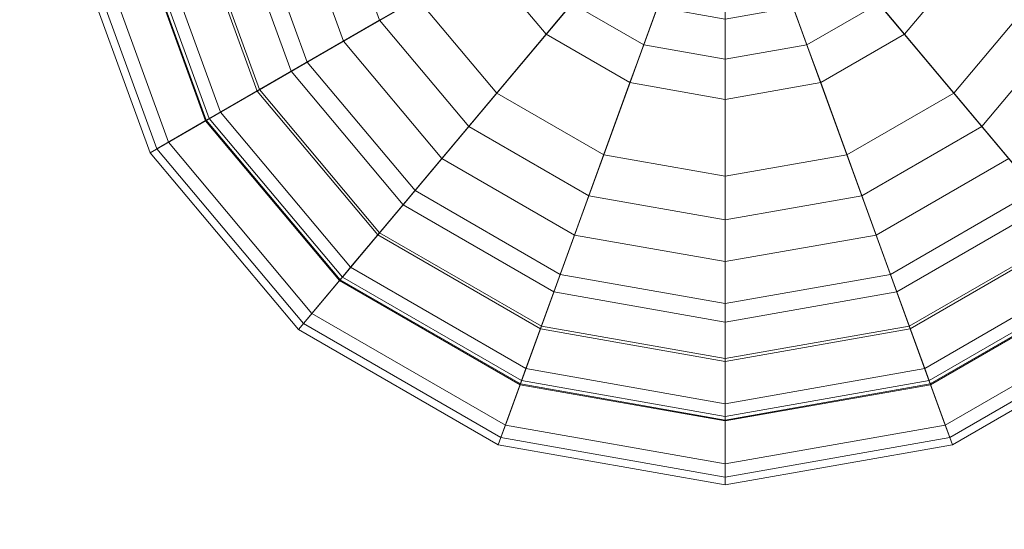
# Model space of a CAD drawing. Units: inches. Extents: x 375 to 1122, y 27 to 1069.
# Tile 90 of 155: x 728.243 to 730.25, y 859.033 to 860.072. Entities that reach past the tile are written whole.
import ezdxf

# ---------------------------------------------------------------- set-up
doc = ezdxf.new("R2010")
doc.units = ezdxf.units.IN
doc.layers.add('A-ANNO-DIMS', color=2, linetype='Continuous', lineweight=18)
doc.layers.add('Furniture', color=30, linetype='Continuous', lineweight=18)
doc.styles.get("Standard").update_dxf_attribs({"font": 'arial.ttf'})
doc.dimstyles.new('ISO-25', dxfattribs={"dimtxt": 12, "dimasz": 2.5, "dimexe": 1.5, "dimexo": 1.5, "dimtad": 1, "dimdec": 1, "dimlunit": 3, "dimtxsty": 'Standard', "dimblk": 'ARCHTICK', "dimcen": 2.5, "dimadec": 0, "dimazin": 0, "dimtfac": 1, "dimtdec": 1, "dimtmove": 0, "dimatfit": 3, "dimfxl": 1.5, "dimfxlon": 1, "dimarcsym": 0})

# ---------------------------------------------------------------- blocks, each defined once
blk = doc.blocks.new('A$C403C54AD')
for points in [[(1.963274, 1.147718, -0.060915), (1.946342, 1.118392, -0.057836), (1.946342, 1.118392, -0.057836), (1.952223, 1.15174, -0.060915)], [(1.95345, 1.130702, -0.054409), (1.961641, 1.144889, -0.057684), (1.951655, 1.148524, -0.057684), (1.948811, 1.13239, -0.054409)], [(1.972282, 1.140158, -0.060915), (1.946342, 1.118392, -0.057836), (1.946342, 1.118392, -0.057836), (1.963274, 1.147718, -0.060915)], [(1.957231, 1.127529, -0.054409), (1.969781, 1.138059, -0.057684), (1.961641, 1.144889, -0.057684), (1.95345, 1.130702, -0.054409)], [(1.96735, 1.13602, 0.042594), (1.961937, 1.131478, 0.032362), (1.956521, 1.136022, 0.032362), (1.960054, 1.142142, 0.042594)], [(1.978163, 1.129974, -0.060915), (1.946342, 1.118392, -0.057836), (1.946342, 1.118392, -0.057836), (1.972282, 1.140158, -0.060915)], [(1.975094, 1.128857, -0.057684), (1.978163, 1.129974, -0.060915), (1.972282, 1.140158, -0.060915), (1.969781, 1.138059, -0.057684)], [(1.960229, 1.130044, 0.03455), (1.965197, 1.134213, 0.043942), (1.958649, 1.139708, 0.043942), (1.955406, 1.134091, 0.03455)], [(1.975056, 1.128843, 0.102069), (1.977788, 1.129837, 0.088845), (1.971977, 1.139902, 0.088845), (1.96975, 1.138033, 0.102069)], [(1.977788, 1.129837, 0.088845), (1.977153, 1.129606, 0.060603), (1.97146, 1.139468, 0.060603), (1.971977, 1.139902, 0.088845)], [(1.977153, 1.129606, 0.060603), (1.972112, 1.127772, 0.042594), (1.96735, 1.13602, 0.042594), (1.97146, 1.139468, 0.060603)], [(1.956521, 1.136022, 0.032362), (1.951402, 1.127155, 0.024995), (1.9481, 1.128357, 0.024995), (1.949878, 1.13844, 0.032362)], [(1.9597, 1.123254, -0.054409), (1.975094, 1.128857, -0.057684), (1.969781, 1.138059, -0.057684), (1.957231, 1.127529, -0.054409)], [(1.970361, 1.127134, 0.111475), (1.975056, 1.128843, 0.102069), (1.96975, 1.138033, 0.102069), (1.965922, 1.134821, 0.111475)], [(1.974889, 1.128782, 0.088628), (1.972249, 1.127821, 0.101264), (1.967462, 1.136113, 0.101264), (1.969614, 1.137919, 0.088628)], [(1.974271, 1.128557, 0.061088), (1.974889, 1.128782, 0.088628), (1.969614, 1.137919, 0.088628), (1.96911, 1.137496, 0.061088)], [(1.969471, 1.12681, 0.043942), (1.974271, 1.128557, 0.061088), (1.96911, 1.137496, 0.061088), (1.965197, 1.134213, 0.043942)], [(1.972249, 1.127821, 0.101264), (1.967468, 1.126081, 0.111475), (1.963564, 1.132843, 0.111475), (1.967462, 1.136113, 0.101264)], [(1.961937, 1.131478, 0.032362), (1.954094, 1.124896, 0.024995), (1.951402, 1.127155, 0.024995), (1.956521, 1.136022, 0.032362)], [(1.972112, 1.127772, 0.042594), (1.965472, 1.125355, 0.032362), (1.961937, 1.131478, 0.032362), (1.96735, 1.13602, 0.042594)], [(1.967468, 1.126081, 0.111475), (1.970361, 1.127134, 0.111475), (1.965922, 1.134821, 0.111475), (1.963564, 1.132843, 0.111475)], [(1.953163, 1.124116, 0.027913), (1.960229, 1.130044, 0.03455), (1.955406, 1.134091, 0.03455), (1.950795, 1.126103, 0.027913)], [(1.963376, 1.124592, 0.03455), (1.969471, 1.12681, 0.043942), (1.965197, 1.134213, 0.043942), (1.960229, 1.130044, 0.03455)], [(1.965472, 1.125355, 0.032362), (1.955851, 1.121853, 0.024995), (1.954094, 1.124896, 0.024995), (1.961937, 1.131478, 0.032362)], [(1.955663, 1.126213, -0.051544), (1.957231, 1.127529, -0.054409), (1.95345, 1.130702, -0.054409), (1.952426, 1.128929, -0.051544)], [(1.980205, 1.118392, -0.060915), (1.946342, 1.118392, -0.057836), (1.946342, 1.118392, -0.057836), (1.978163, 1.129974, -0.060915)], [(1.95471, 1.121437, 0.027913), (1.963376, 1.124592, 0.03455), (1.960229, 1.130044, 0.03455), (1.953163, 1.124116, 0.027913)], [(1.979131, 1.118392, 0.060603), (1.973766, 1.118392, 0.042594), (1.972112, 1.127772, 0.042594), (1.977153, 1.129606, 0.060603)], [(1.976898, 1.118392, 0.102069), (1.979806, 1.118392, 0.088845), (1.977788, 1.129837, 0.088845), (1.975056, 1.128843, 0.102069)], [(1.976939, 1.118392, -0.057684), (1.980205, 1.118392, -0.060915), (1.978163, 1.129974, -0.060915), (1.975094, 1.128857, -0.057684)], [(1.979806, 1.118392, 0.088845), (1.979131, 1.118392, 0.060603), (1.977153, 1.129606, 0.060603), (1.977788, 1.129837, 0.088845)], [(1.960557, 1.118392, -0.054409), (1.976939, 1.118392, -0.057684), (1.975094, 1.128857, -0.057684), (1.9597, 1.123254, -0.054409)], [(1.971902, 1.118392, 0.111475), (1.976898, 1.118392, 0.102069), (1.975056, 1.128843, 0.102069), (1.970361, 1.127134, 0.111475)], [(1.976721, 1.118392, 0.088628), (1.973912, 1.118392, 0.101264), (1.972249, 1.127821, 0.101264), (1.974889, 1.128782, 0.088628)], [(1.976063, 1.118392, 0.061088), (1.976721, 1.118392, 0.088628), (1.974889, 1.128782, 0.088628), (1.974271, 1.128557, 0.061088)], [(1.970956, 1.118392, 0.043942), (1.976063, 1.118392, 0.061088), (1.974271, 1.128557, 0.061088), (1.969471, 1.12681, 0.043942)], [(1.973766, 1.118392, 0.042594), (1.9667, 1.118392, 0.032362), (1.965472, 1.125355, 0.032362), (1.972112, 1.127772, 0.042594)], [(1.973912, 1.118392, 0.101264), (1.968824, 1.118392, 0.111475), (1.967468, 1.126081, 0.111475), (1.972249, 1.127821, 0.101264)], [(1.957775, 1.122553, -0.051544), (1.9597, 1.123254, -0.054409), (1.957231, 1.127529, -0.054409), (1.955663, 1.126213, -0.051544)], [(1.968824, 1.118392, 0.111475), (1.971902, 1.118392, 0.111475), (1.970361, 1.127134, 0.111475), (1.967468, 1.126081, 0.111475)], [(1.96447, 1.118392, 0.03455), (1.970956, 1.118392, 0.043942), (1.969471, 1.12681, 0.043942), (1.963376, 1.124592, 0.03455)], [(1.953927, 1.121153, -0.049498), (1.957775, 1.122553, -0.051544), (1.955663, 1.126213, -0.051544), (1.952525, 1.12358, -0.049498)], [(1.9667, 1.118392, 0.032362), (1.956461, 1.118392, 0.024995), (1.955851, 1.121853, 0.024995), (1.965472, 1.125355, 0.032362)], [(1.955247, 1.118392, 0.027913), (1.96447, 1.118392, 0.03455), (1.963376, 1.124592, 0.03455), (1.95471, 1.121437, 0.027913)], [(1.958509, 1.118392, -0.051544), (1.960557, 1.118392, -0.054409), (1.9597, 1.123254, -0.054409), (1.957775, 1.122553, -0.051544)], [(1.954413, 1.118392, -0.049498), (1.958509, 1.118392, -0.051544), (1.957775, 1.122553, -0.051544), (1.953927, 1.121153, -0.049498)], [(1.972282, 1.096626, -0.060915), (1.946342, 1.118392, -0.057836), (1.946342, 1.118392, -0.057836), (1.978163, 1.106811, -0.060915)], [(1.963274, 1.089067, -0.060915), (1.946342, 1.118392, -0.057836), (1.946342, 1.118392, -0.057836), (1.972282, 1.096626, -0.060915)], [(1.952223, 1.085044, -0.060915), (1.946342, 1.118392, -0.057836), (1.946342, 1.118392, -0.057836), (1.963274, 1.089067, -0.060915)], [(1.978163, 1.106811, -0.060915), (1.946342, 1.118392, -0.057836), (1.946342, 1.118392, -0.057836), (1.980205, 1.118392, -0.060915)], [(1.953927, 1.115632, -0.049498), (1.957775, 1.114231, -0.051544), (1.958509, 1.118392, -0.051544), (1.954413, 1.118392, -0.049498)], [(1.95471, 1.115347, 0.027913), (1.963376, 1.112192, 0.03455), (1.96447, 1.118392, 0.03455), (1.955247, 1.118392, 0.027913)], [(1.965472, 1.111429, 0.032362), (1.955851, 1.114931, 0.024995), (1.956461, 1.118392, 0.024995), (1.9667, 1.118392, 0.032362)], [(1.957775, 1.114231, -0.051544), (1.9597, 1.113531, -0.054409), (1.960557, 1.118392, -0.054409), (1.958509, 1.118392, -0.051544)], [(1.9597, 1.113531, -0.054409), (1.975094, 1.107928, -0.057684), (1.976939, 1.118392, -0.057684), (1.960557, 1.118392, -0.054409)], [(1.963376, 1.112192, 0.03455), (1.969471, 1.109974, 0.043942), (1.970956, 1.118392, 0.043942), (1.96447, 1.118392, 0.03455)], [(1.972112, 1.109013, 0.042594), (1.965472, 1.111429, 0.032362), (1.9667, 1.118392, 0.032362), (1.973766, 1.118392, 0.042594)], [(1.967468, 1.110703, 0.111475), (1.970361, 1.10965, 0.111475), (1.971902, 1.118392, 0.111475), (1.968824, 1.118392, 0.111475)], [(1.972249, 1.108963, 0.101264), (1.967468, 1.110703, 0.111475), (1.968824, 1.118392, 0.111475), (1.973912, 1.118392, 0.101264)], [(1.969471, 1.109974, 0.043942), (1.974271, 1.108227, 0.061088), (1.976063, 1.118392, 0.061088), (1.970956, 1.118392, 0.043942)], [(1.970361, 1.10965, 0.111475), (1.975056, 1.107941, 0.102069), (1.976898, 1.118392, 0.102069), (1.971902, 1.118392, 0.111475)], [(1.977153, 1.107178, 0.060603), (1.972112, 1.109013, 0.042594), (1.973766, 1.118392, 0.042594), (1.979131, 1.118392, 0.060603)], [(1.974889, 1.108002, 0.088628), (1.972249, 1.108963, 0.101264), (1.973912, 1.118392, 0.101264), (1.976721, 1.118392, 0.088628)], [(1.974271, 1.108227, 0.061088), (1.974889, 1.108002, 0.088628), (1.976721, 1.118392, 0.088628), (1.976063, 1.118392, 0.061088)], [(1.975056, 1.107941, 0.102069), (1.977788, 1.106947, 0.088845), (1.979806, 1.118392, 0.088845), (1.976898, 1.118392, 0.102069)], [(1.975094, 1.107928, -0.057684), (1.978163, 1.106811, -0.060915), (1.980205, 1.118392, -0.060915), (1.976939, 1.118392, -0.057684)], [(1.977788, 1.106947, 0.088845), (1.977153, 1.107178, 0.060603), (1.979131, 1.118392, 0.060603), (1.979806, 1.118392, 0.088845)], [(1.952525, 1.113204, -0.049498), (1.955663, 1.110572, -0.051544), (1.957775, 1.114231, -0.051544), (1.953927, 1.115632, -0.049498)], [(1.953163, 1.112669, 0.027913), (1.960229, 1.10674, 0.03455), (1.963376, 1.112192, 0.03455), (1.95471, 1.115347, 0.027913)], [(1.961937, 1.105307, 0.032362), (1.954094, 1.111888, 0.024995), (1.955851, 1.114931, 0.024995), (1.965472, 1.111429, 0.032362)], [(1.955663, 1.110572, -0.051544), (1.957231, 1.109255, -0.054409), (1.9597, 1.113531, -0.054409), (1.957775, 1.114231, -0.051544)], [(1.957231, 1.109255, -0.054409), (1.969781, 1.098725, -0.057684), (1.975094, 1.107928, -0.057684), (1.9597, 1.113531, -0.054409)], [(1.950795, 1.110681, 0.027913), (1.955406, 1.102693, 0.03455), (1.960229, 1.10674, 0.03455), (1.953163, 1.112669, 0.027913)], [(1.960229, 1.10674, 0.03455), (1.965197, 1.102571, 0.043942), (1.969471, 1.109974, 0.043942), (1.963376, 1.112192, 0.03455)], [(1.956521, 1.100762, 0.032362), (1.951402, 1.109629, 0.024995), (1.954094, 1.111888, 0.024995), (1.961937, 1.105307, 0.032362)], [(1.96735, 1.100764, 0.042594), (1.961937, 1.105307, 0.032362), (1.965472, 1.111429, 0.032362), (1.972112, 1.109013, 0.042594)], [(1.952426, 1.107856, -0.051544), (1.95345, 1.106082, -0.054409), (1.957231, 1.109255, -0.054409), (1.955663, 1.110572, -0.051544)], [(1.963564, 1.103941, 0.111475), (1.965922, 1.101963, 0.111475), (1.970361, 1.10965, 0.111475), (1.967468, 1.110703, 0.111475)], [(1.967462, 1.100671, 0.101264), (1.963564, 1.103941, 0.111475), (1.967468, 1.110703, 0.111475), (1.972249, 1.108963, 0.101264)], [(1.949878, 1.098344, 0.032362), (1.9481, 1.108427, 0.024995), (1.951402, 1.109629, 0.024995), (1.956521, 1.100762, 0.032362)], [(1.965197, 1.102571, 0.043942), (1.96911, 1.099288, 0.061088), (1.974271, 1.108227, 0.061088), (1.969471, 1.109974, 0.043942)], [(1.965922, 1.101963, 0.111475), (1.96975, 1.098751, 0.102069), (1.975056, 1.107941, 0.102069), (1.970361, 1.10965, 0.111475)], [(1.95345, 1.106082, -0.054409), (1.961641, 1.091895, -0.057684), (1.969781, 1.098725, -0.057684), (1.957231, 1.109255, -0.054409)], [(1.97146, 1.097316, 0.060603), (1.96735, 1.100764, 0.042594), (1.972112, 1.109013, 0.042594), (1.977153, 1.107178, 0.060603)], [(1.969614, 1.098865, 0.088628), (1.967462, 1.100671, 0.101264), (1.972249, 1.108963, 0.101264), (1.974889, 1.108002, 0.088628)], [(1.96911, 1.099288, 0.061088), (1.969614, 1.098865, 0.088628), (1.974889, 1.108002, 0.088628), (1.974271, 1.108227, 0.061088)], [(1.96975, 1.098751, 0.102069), (1.971977, 1.096882, 0.088845), (1.977788, 1.106947, 0.088845), (1.975056, 1.107941, 0.102069)], [(1.969781, 1.098725, -0.057684), (1.972282, 1.096626, -0.060915), (1.978163, 1.106811, -0.060915), (1.975094, 1.107928, -0.057684)], [(1.971977, 1.096882, 0.088845), (1.97146, 1.097316, 0.060603), (1.977153, 1.107178, 0.060603), (1.977788, 1.106947, 0.088845)], [(1.955406, 1.102693, 0.03455), (1.958649, 1.097077, 0.043942), (1.965197, 1.102571, 0.043942), (1.960229, 1.10674, 0.03455)], [(1.948811, 1.104394, -0.054409), (1.951655, 1.088261, -0.057684), (1.961641, 1.091895, -0.057684), (1.95345, 1.106082, -0.054409)], [(1.960054, 1.094642, 0.042594), (1.956521, 1.100762, 0.032362), (1.961937, 1.105307, 0.032362), (1.96735, 1.100764, 0.042594)], [(1.957583, 1.098923, 0.111475), (1.959122, 1.096257, 0.111475), (1.965922, 1.101963, 0.111475), (1.963564, 1.103941, 0.111475)], [(1.960127, 1.094517, 0.101264), (1.957583, 1.098923, 0.111475), (1.963564, 1.103941, 0.111475), (1.967462, 1.100671, 0.101264)], [(1.94949, 1.10054, 0.03455), (1.950616, 1.094153, 0.043942), (1.958649, 1.097077, 0.043942), (1.955406, 1.102693, 0.03455)], [(1.958649, 1.097077, 0.043942), (1.961203, 1.092653, 0.061088), (1.96911, 1.099288, 0.061088), (1.965197, 1.102571, 0.043942)], [(1.959122, 1.096257, 0.111475), (1.96162, 1.09193, 0.102069), (1.96975, 1.098751, 0.102069), (1.965922, 1.101963, 0.111475)], [(1.951105, 1.091385, 0.042594), (1.949878, 1.098344, 0.032362), (1.956521, 1.100762, 0.032362), (1.960054, 1.094642, 0.042594)], [(1.962737, 1.089997, 0.060603), (1.960054, 1.094642, 0.042594), (1.96735, 1.100764, 0.042594), (1.97146, 1.097316, 0.060603)], [(1.961532, 1.092083, 0.088628), (1.960127, 1.094517, 0.101264), (1.967462, 1.100671, 0.101264), (1.969614, 1.098865, 0.088628)], [(1.961203, 1.092653, 0.061088), (1.961532, 1.092083, 0.088628), (1.969614, 1.098865, 0.088628), (1.96911, 1.099288, 0.061088)], [(1.950246, 1.096252, 0.111475), (1.950781, 1.093221, 0.111475), (1.959122, 1.096257, 0.111475), (1.957583, 1.098923, 0.111475)], [(1.95113, 1.091242, 0.101264), (1.950246, 1.096252, 0.111475), (1.957583, 1.098923, 0.111475), (1.960127, 1.094517, 0.101264)], [(1.96162, 1.09193, 0.102069), (1.963074, 1.089412, 0.088845), (1.971977, 1.096882, 0.088845), (1.96975, 1.098751, 0.102069)], [(1.961641, 1.091895, -0.057684), (1.963274, 1.089067, -0.060915), (1.972282, 1.096626, -0.060915), (1.969781, 1.098725, -0.057684)], [(1.950616, 1.094153, 0.043942), (1.951503, 1.089123, 0.061088), (1.961203, 1.092653, 0.061088), (1.958649, 1.097077, 0.043942)], [(1.963074, 1.089412, 0.088845), (1.962737, 1.089997, 0.060603), (1.97146, 1.097316, 0.060603), (1.971977, 1.096882, 0.088845)], [(1.950781, 1.093221, 0.111475), (1.951648, 1.0883, 0.102069), (1.96162, 1.09193, 0.102069), (1.959122, 1.096257, 0.111475)], [(1.952036, 1.086102, 0.060603), (1.951105, 1.091385, 0.042594), (1.960054, 1.094642, 0.042594), (1.962737, 1.089997, 0.060603)], [(1.951618, 1.088475, 0.088628), (1.95113, 1.091242, 0.101264), (1.960127, 1.094517, 0.101264), (1.961532, 1.092083, 0.088628)], [(1.951503, 1.089123, 0.061088), (1.951618, 1.088475, 0.088628), (1.961532, 1.092083, 0.088628), (1.961203, 1.092653, 0.061088)], [(1.951648, 1.0883, 0.102069), (1.952153, 1.085437, 0.088845), (1.963074, 1.089412, 0.088845), (1.96162, 1.09193, 0.102069)], [(1.951655, 1.088261, -0.057684), (1.952223, 1.085044, -0.060915), (1.963274, 1.089067, -0.060915), (1.961641, 1.091895, -0.057684)], [(1.952153, 1.085437, 0.088845), (1.952036, 1.086102, 0.060603), (1.962737, 1.089997, 0.060603), (1.963074, 1.089412, 0.088845)]]:
    blk.add_3dface(points)
at = {"linetype": 'ByBlock', "invisible_edges": 5}
for points in [[(1.994146, 1.087608, -0.037827), (2.010142, 1.078373, -0.037827), (1.994057, 1.018345, -0.037827), (1.975587, 1.018345, -0.037827)], [(2.023472, 1.070677, -0.05168), (1.994146, 1.087608, -0.042444), (1.975587, 1.018345, -0.042444), (2.009449, 1.018345, -0.05168)]]:
    blk.add_3dface(points, dxfattribs=at)
at = {"linetype": 'ByBlock'}
blk.add_3dface([(1.994146, 1.087608, -0.042444), (1.994146, 1.087608, -0.037827), (1.975587, 1.018345, -0.037827), (1.975587, 1.018345, -0.042444)], dxfattribs=at)
blk = doc.blocks.new('_ArchTick')
at = {"color": 0, "linetype": 'ByBlock', "const_width": 0.15}
blk.add_lwpolyline([(-0.5, -0.5), (0.5, 0.5)], dxfattribs=at)
blk = doc.blocks.new('*D85')
at = {"layer": 'A-ANNO-DIMS', "color": 0, "lineweight": -2, "transparency": 16777216}
for p, q in [((401.5073, 868.5277), (398.5073, 868.5277)), ((400.0073, 814.5277), (400.0073, 868.5277)), ((401.5073, 814.5277), (398.5073, 814.5277))]:
    blk.add_line(p, q, dxfattribs=at)
at = {"layer": 'Defpoints', "color": 0, "transparency": 16777216}
for p in [(400.0073, 868.5277), (845.0073, 868.5277), (845.0073, 814.5277)]:
    blk.add_point(p, dxfattribs=at)
at = {"layer": 'A-ANNO-DIMS', "color": 0, "lineweight": -2, "transparency": 16777216, "xscale": 2.5, "yscale": 2.5, "zscale": 2.5}
for p, rotation in [((400.0073, 868.5277), 90), ((400.0073, 814.5277), 270)]:
    blk.add_blockref('_ArchTick', p, dxfattribs=dict(at, rotation=rotation))
at = {"layer": 'A-ANNO-DIMS', "color": 0, "transparency": 16777216, "insert": (393.2555, 841.5277), "char_height": 12, "attachment_point": 5, "rotation": 90}
blk.add_mtext('4\'-6"', dxfattribs=at)
blk = doc.blocks.new('*D88')
at = {"layer": 'A-ANNO-DIMS', "color": 0, "lineweight": -2, "transparency": 16777216}
for p, q in [((731.0073, 1052.5277), (731.0073, 1055.5277)), ((854.0073, 1052.5277), (854.0073, 1055.5277)), ((731.0073, 1054.0277), (854.0073, 1054.0277))]:
    blk.add_line(p, q, dxfattribs=at)
at = {"layer": 'Defpoints', "color": 0, "transparency": 16777216}
for p in [(854.0073, 1054.0277), (731.0073, 502.5277), (854.0073, 502.5277)]:
    blk.add_point(p, dxfattribs=at)
at = {"layer": 'A-ANNO-DIMS', "color": 0, "lineweight": -2, "transparency": 16777216, "xscale": 2.5, "yscale": 2.5, "zscale": 2.5, "rotation": 180}
blk.add_blockref('_ArchTick', (731.0073, 1054.0277), dxfattribs=at)
at = {"layer": 'A-ANNO-DIMS', "color": 0, "lineweight": -2, "transparency": 16777216, "xscale": 2.5, "yscale": 2.5, "zscale": 2.5}
blk.add_blockref('_ArchTick', (854.0073, 1054.0277), dxfattribs=at)
at = {"layer": 'A-ANNO-DIMS', "color": 0, "transparency": 16777216, "insert": (792.5073, 1060.7837), "char_height": 12, "attachment_point": 5}
blk.add_mtext('10\'-3"', dxfattribs=at)
blk = doc.blocks.new('*D91')
at = {"layer": 'A-ANNO-DIMS', "color": 0, "lineweight": -2, "transparency": 16777216}
for p, q in [((728.0073, 1052.5277), (728.0073, 1055.5277)), ((788.0073, 1052.5277), (788.0073, 1055.5277)), ((728.0073, 1054.0277), (788.0073, 1054.0277))]:
    blk.add_line(p, q, dxfattribs=at)
at = {"layer": 'Defpoints', "color": 0, "transparency": 16777216}
for p in [(788.0073, 1054.0277), (728.0073, 774.0277), (788.0073, 774.0277)]:
    blk.add_point(p, dxfattribs=at)
at = {"layer": 'A-ANNO-DIMS', "color": 0, "lineweight": -2, "transparency": 16777216, "xscale": 2.5, "yscale": 2.5, "zscale": 2.5, "rotation": 180}
blk.add_blockref('_ArchTick', (728.0073, 1054.0277), dxfattribs=at)
at = {"layer": 'A-ANNO-DIMS', "color": 0, "lineweight": -2, "transparency": 16777216, "xscale": 2.5, "yscale": 2.5, "zscale": 2.5}
blk.add_blockref('_ArchTick', (788.0073, 1054.0277), dxfattribs=at)
at = {"layer": 'A-ANNO-DIMS', "color": 0, "transparency": 16777216, "insert": (758.0073, 1060.7796), "char_height": 12, "attachment_point": 5}
blk.add_mtext('5\'-0"', dxfattribs=at)

msp = doc.modelspace()

# ---------------------------------------------------------------- block references
at = {"layer": 'Furniture', "xscale": 39.9918517141215, "yscale": 39.9918517141215, "zscale": 39.9918517141215, "rotation": 270}
msp.add_blockref('A$C403C54AD', (684.9549, 938.3156, 0.024), dxfattribs=at)

# ---------------------------------------------------------------- dimensions: what is measured, and where the dimension line sits
at = {"layer": 'A-ANNO-DIMS'}
for base, p1, p2, picture, middle in [((788.0073, 1054.0277), (728.0073, 774.0277), (788.0073, 774.0277), '*D91', (758.0073, 1060.7796)), ((854.0073, 1054.0277), (731.0073, 502.5277), (854.0073, 502.5277), '*D88', (792.5073, 1060.7837))]:
    dim = msp.add_linear_dim(base=base, p1=p1, p2=p2, dimstyle='ISO-25', override={"dimdec": 1, "dimlfac": 1, "dimrnd": 0, "dimzin": 1, "dimdsep": 46, "dimlunit": 4, "dimfrac": 2}, dxfattribs=at)
    dim.commit()
    dim.dimension.update_dxf_attribs({"geometry": picture, "text_midpoint": middle})
dim = msp.add_linear_dim(base=(400.0073, 868.5277), p1=(845.0073, 814.5277), p2=(845.0073, 868.5277), angle=90, dimstyle='ISO-25', override={"dimdec": 1, "dimlfac": 1, "dimrnd": 0, "dimzin": 1, "dimdsep": 46, "dimlunit": 4, "dimfrac": 2}, dxfattribs=at)
dim.commit()
dim.dimension.update_dxf_attribs({"geometry": '*D85', "text_midpoint": (393.2555, 841.5277)})

doc.saveas('drawing.dxf')
